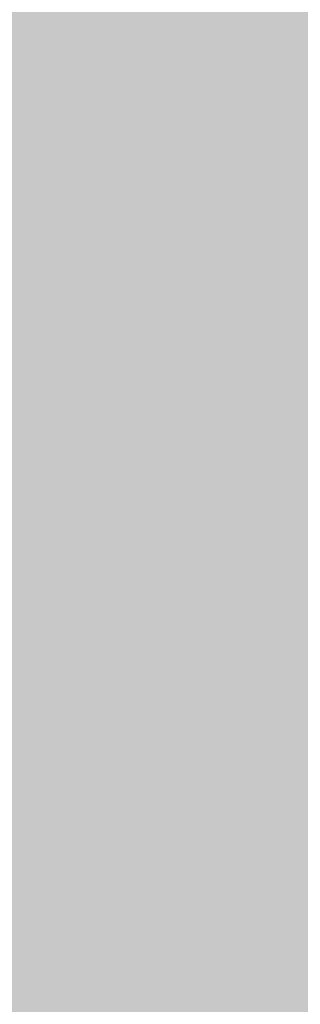
# Model space of a CAD drawing. Units: inches. Extents: x 2083 to 3317, y 1141 to 2115.
# Tile 178 of 256: x 3126.92826 to 3126.94671, y 1263.29018 to 1263.35483. Entities that reach past the tile are written whole.
import ezdxf

# ---------------------------------------------------------------- set-up
doc = ezdxf.new("R2010")
doc.units = ezdxf.units.IN
doc.layers.add('A-ANNO-DIMS', color=2, linetype='Continuous', lineweight=18)
doc.layers.add('A-WALL-PATT', color=251, linetype='Continuous', lineweight=13, true_color=0x636466)
doc.styles.get("Standard").update_dxf_attribs({"font": 'arial.ttf'})
doc.dimstyles.new('ISO-25', dxfattribs={"dimtxt": 12, "dimasz": 12, "dimexe": 1.25, "dimexo": 0.625, "dimtad": 1, "dimlunit": 3, "dimtxsty": 'Standard', "dimcen": 2.5, "dimadec": 0, "dimazin": 0, "dimtfac": 1, "dimtmove": 0, "dimatfit": 3, "dimfxl": 1, "dimarcsym": 0})

# ---------------------------------------------------------------- blocks, each defined once
blk = doc.blocks.new('*D26')
at = {"layer": 'A-ANNO-DIMS', "color": 0, "lineweight": -2, "transparency": 16777216}
for p, q in [((3088.985844, 1274.915092), (3088.985844, 1270.951963)), ((3111.240037, 1274.915092), (3111.240037, 1270.951963)), ((3076.985844, 1272.201963), (2840.262447, 1272.201963)), ((3111.240037, 1272.201963), (3088.985844, 1272.201963)), ((3123.240037, 1272.201963), (3135.240037, 1272.201963))]:
    blk.add_line(p, q, dxfattribs=at)
at = {"layer": 'A-ANNO-DIMS', "color": 0, "transparency": 16777216}
for points in [[(3076.985844, 1274.201963), (3076.985844, 1270.201963), (3088.985844, 1272.201963)], [(3123.240037, 1274.201963), (3123.240037, 1270.201963), (3111.240037, 1272.201963)]]:
    blk.add_solid(points, dxfattribs=at)
at = {"layer": 'Defpoints', "color": 0, "transparency": 16777216}
for p in [(3088.985844, 1275.540092), (3111.240037, 1275.540092), (3088.985844, 1272.201963)]:
    blk.add_point(p, dxfattribs=at)
at = {"layer": 'A-ANNO-DIMS', "color": 0, "transparency": 16777216, "insert": (2952.624146, 1279.031602), "char_height": 12, "attachment_point": 5}
blk.add_mtext('NIGHTSTAND 1\'-10 1/2" TYP.', dxfattribs=at)
blk = doc.blocks.new('*D27')
at = {"layer": 'A-ANNO-DIMS', "color": 0, "lineweight": -2, "transparency": 16777216}
for p, q in [((3114.578165, 1309.794285), (3114.578165, 1321.794285)), ((3111.865037, 1297.794285), (3115.828165, 1297.794285)), ((3114.578165, 1297.794285), (3114.578165, 1275.540092)), ((3111.865037, 1275.540092), (3115.828165, 1275.540092)), ((3114.578165, 1263.540092), (3114.578165, 1140.988591))]:
    blk.add_line(p, q, dxfattribs=at)
at = {"layer": 'A-ANNO-DIMS', "color": 0, "transparency": 16777216}
for points in [[(3112.578165, 1309.794285), (3116.578165, 1309.794285), (3114.578165, 1297.794285)], [(3112.578165, 1263.540092), (3116.578165, 1263.540092), (3114.578165, 1275.540092)]]:
    blk.add_solid(points, dxfattribs=at)
at = {"layer": 'Defpoints', "color": 0, "transparency": 16777216}
for p in [(3111.240037, 1297.794285), (3111.240037, 1275.540092), (3114.578165, 1275.540092)]:
    blk.add_point(p, dxfattribs=at)
at = {"layer": 'A-ANNO-DIMS', "color": 0, "transparency": 16777216, "insert": (3107.748527, 1196.264342), "char_height": 12, "attachment_point": 5, "rotation": 90}
blk.add_mtext('1\'-10 1/2" TYP.', dxfattribs=at)

msp = doc.modelspace()

# ---------------------------------------------------------------- hatches: boundary and pattern name
at = {"layer": 'A-WALL-PATT'}
h = msp.add_hatch(color=256, dxfattribs=at)
h.dxf.hatch_style = 1
h.paths.add_polyline_path([(3126.959783, 2020.76136), (2748.959783, 2020.76136), (2604.959783, 2020.76136), (2226.959783, 2020.76136), (2226.959783, 1702.76136), (2466.959783, 1702.76136), (2466.959783, 1582.76136), (2418.959783, 1582.76136), (2418.959783, 1477.76136), (2226.959783, 1477.76136), (2226.959783, 1263.26136), (2544.959783, 1263.26136), (2544.959783, 1411.76136), (2604.959783, 1411.76136), (2685.959783, 1411.76136), (2685.959783, 1420.76136), (2604.959783, 1420.76136), (2604.959783, 1573.76136), (2604.959783, 1702.76136), (2604.959783, 2011.76136), (2748.959783, 2011.76136), (2748.959783, 1702.76136), (2862.959783, 1702.76136), (2862.959783, 1621.76136), (2871.959783, 1621.76136), (2871.959783, 1702.76136), (2883.959783, 1702.76136), (2883.959783, 1706.939459, -0.026459), (2883.959783, 1711.76136), (2757.959783, 1711.76136), (2757.959783, 1807.76136), (2787.959783, 1807.76136), (2787.959783, 1812.26136), (2757.959783, 1812.26136), (2757.959783, 2011.76136), (2877.959783, 2011.76136), (2877.959783, 1812.26136), (2847.959783, 1812.26136), (2847.959783, 1807.76136), (2889.835742, 1807.76136), (2889.835742, 1812.26136), (2882.459783, 1812.26136), (2882.459783, 2011.76136), (3117.959783, 2011.76136), (3117.959783, 1812.26136), (2937.835742, 1812.26136), (2937.835742, 1807.76136), (2995.709783, 1807.76136), (2995.709783, 1796.117666), (3000.209783, 1796.117666), (3000.209783, 1807.76136), (3117.959783, 1807.76136), (3117.959783, 1711.76136), (3000.209783, 1711.76136), (3000.209783, 1760.117666), (2998.572705, 1760.117666, -0.020711), (2995.709783, 1760.117666), (2995.709783, 1711.76136), (2931.959783, 1711.76136), (2931.959783, 1702.76136), (3126.959783, 1702.76136)])
h.paths.add_polyline_path([(2471.459783, 2011.76136), (2471.459783, 1810.01136), (2462.716936, 1810.01136), (2462.716936, 1805.51136), (2505.959783, 1805.51136), (2505.959783, 1810.01136), (2475.959783, 1810.01136), (2475.959783, 2011.76136), (2595.959783, 2011.76136), (2595.959783, 1810.01136), (2565.959783, 1810.01136), (2565.959783, 1805.51136), (2595.959783, 1805.51136), (2595.959783, 1711.76136), (2235.959783, 1711.76136), (2235.959783, 1805.51136), (2353.709783, 1805.51136), (2353.709783, 1796.054162), (2358.209783, 1796.054162), (2358.209783, 1805.51136), (2414.716936, 1805.51136), (2414.716936, 1810.01136), (2235.959783, 1810.01136), (2235.959783, 2011.76136)], flags=16)
h.paths.add_polyline_path([(2270.204734, 1994.610008), (2270.204734, 1970.610008), (2246.204734, 1970.610008), (2246.204734, 1994.610008)], flags=0)
edge = h.paths.add_edge_path(flags=0)
edge.add_ellipse((2332.027391, 1899.798176), major_axis=(-3.042994, 3.042994), ratio=0.16825245, start_angle=-161.332166, end_angle=-156.307114, ccw=False)
edge.add_ellipse((2333.082037, 1898.74353), major_axis=(-1.054646, 1.054646), ratio=0.4535321, start_angle=-123.371019, end_angle=-94.159107)
edge = h.paths.add_edge_path(flags=0)
edge.add_ellipse((2332.027391, 1968.87629), major_axis=(3.042994, 3.042994), ratio=0.16825245, start_angle=18.667834, end_angle=23.692886)
edge.add_spline(control_points=[(2332.925596, 1970.691105), (2332.226768, 1970.3361), (2330.893709, 1969.658905), (2328.41308, 1970.932138), (2327.203934, 1967.748712), (2324.709596, 1969.955589), (2322.532822, 1967.012354), (2320.012846, 1971.295812), (2317.680308, 1968.157845), (2316.040526, 1967.102047), (2315.426904, 1966.809602)], knot_values=[0, 0, 0, 0, 2.267059, 4.324559, 6.685584, 8.878641, 11.121502, 14.300359, 17.755284, 19.732645, 19.732645, 19.732645, 19.732645], degree=3, periodic=0)
edge.add_ellipse((2332.027391, 1968.87629), major_axis=(3.042994, 3.042994), ratio=0.16825245, start_angle=18.667834, end_angle=23.692886, ccw=False)
edge.add_ellipse((2333.082037, 1969.930936), major_axis=(1.054646, 1.054646), ratio=0.4535321, start_angle=56.628981, end_angle=85.840893, ccw=False)
edge = h.paths.add_edge_path(flags=0)
edge.add_spline(control_points=[(2296.428287, 1967.987908), (2293.627804, 1965.336314), (2287.703624, 1959.727094), (2299.74386, 1949.995699), (2294.532591, 1935.668528), (2290.573228, 1920.603512), (2293.394124, 1909.973691), (2296.185407, 1904.966543)], knot_values=[0.099185, 0.099185, 0.099185, 0.099185, 0.345301, 0.619822, 0.982653, 1.386093, 1.810555, 1.810555, 1.810555, 1.810555], degree=3, periodic=0)
edge.add_spline(control_points=[(2296.185407, 1904.966543), (2297.383582, 1902.6193), (2298.000969, 1901.949312), (2298.55297, 1901.468155)], knot_values=[0.006246, 0.006246, 0.006246, 0.006246, 0.055476, 0.055476, 0.055476, 0.055476], degree=3, periodic=0)
edge.add_spline(control_points=[(2298.55297, 1901.468155), (2297.258612, 1900.923224), (2295.225294, 1900.232126), (2293.060229, 1900.614205), (2292.101423, 1900.788415), (2292.089578, 1900.790568)], knot_values=[0.312835, 0.312835, 0.312835, 0.312835, 0.40178, 0.474987, 0.475903, 0.475903, 0.475903, 0.475903], degree=3, periodic=0)
edge.add_arc((2292.793646, 1904.664109), 3.937008, 215.420897, 259.698179, ccw=False)
edge.add_spline(control_points=[(2289.585314, 1902.382304), (2289.476652, 1902.535087), (2289.36848, 1902.688035), (2289.260865, 1902.84117)], knot_values=[0.102872, 0.102872, 0.102872, 0.102872, 0.116896, 0.116896, 0.116896, 0.116896], degree=3, periodic=0)
edge.add_spline(control_points=[(2289.260865, 1902.84117), (2288.686604, 1902.550192), (2287.640048, 1902.019902), (2285.881337, 1901.873954), (2283.852972, 1901.504352), (2281.719987, 1899.710538), (2278.466991, 1899.492942), (2276.157136, 1901.883202), (2272.258953, 1899.804071), (2267.777605, 1901.843183), (2262.243882, 1900.184033), (2257.414927, 1901.782061), (2254.318374, 1900.72612), (2253.178285, 1900.337343)], knot_values=[0, 0, 0, 0, 1.907977, 3.477176, 5.261074, 7.972851, 11.680248, 13.717921, 16.939592, 22.789562, 27.502503, 33.595215, 37.145618, 37.145618, 37.145618, 37.145618], degree=3, periodic=0)
edge.add_line((2253.178285, 1900.337343), (2250.24424, 1902.84117))
edge.add_line((2250.24424, 1902.84117), (2250.24424, 1965.833296))
edge.add_line((2250.24424, 1965.833296), (2253.178285, 1968.337123))
edge.add_spline(control_points=[(2253.178285, 1968.337123), (2254.318374, 1967.948346), (2257.414927, 1966.892405), (2262.243882, 1968.490433), (2267.777605, 1966.831283), (2271.52673, 1968.537217), (2273.875914, 1967.828289), (2274.206701, 1967.727642)], knot_values=[0, 0, 0, 0, 0.09018, 0.244935, 0.364644, 0.513233, 0.537855, 0.537855, 0.537855, 0.537855], degree=3, periodic=0)
edge.add_arc((2274.352887, 1963.793349), 3.937008, 72.051134, 92.127949, ccw=False)
edge.add_arc((2281.296933, 1985.230003), 18.596298, 252.0511336, 288.5657217)
edge.add_arc((2292.316717, 1956.02888), 12.646081, 71.0267879, 113.7782184, ccw=False)
edge = h.paths.add_edge_path(flags=0)
edge.add_spline(control_points=[(2274.899415, 1951.856195), (2275.066156, 1951.616592), (2275.232687, 1951.376588), (2275.397987, 1951.135855)], knot_values=[1.409916, 1.409916, 1.409916, 1.409916, 1.43159, 1.43159, 1.43159, 1.43159], degree=3, periodic=0)
edge.add_spline(control_points=[(2275.397987, 1951.135855), (2275.792106, 1950.561885), (2276.179231, 1949.983774), (2276.545546, 1949.397103)], knot_values=[1.358238, 1.358238, 1.358238, 1.358238, 1.409916, 1.409916, 1.409916, 1.409916], degree=3, periodic=0)
edge.add_line((2276.545546, 1949.397103), (2277.437289, 1947.862185))
edge.add_spline(control_points=[(2277.437289, 1947.862185), (2276.303834, 1945.673115), (2274.639698, 1942.426882), (2274.631615, 1938.0939), (2272.799124, 1930.85155), (2274.356426, 1943.897046), (2275.947681, 1947.923356), (2276.545546, 1949.397103)], knot_values=[0.005632, 0.005632, 0.005632, 0.005632, 0.186014, 0.266002, 0.357087, 0.59639, 0.739732, 0.739732, 0.739732, 0.739732], degree=3, periodic=0)
edge.add_spline(control_points=[(2276.545546, 1949.397103), (2276.179231, 1949.983774), (2275.792106, 1950.561885), (2275.397987, 1951.135855)], knot_values=[1.358238, 1.358238, 1.358238, 1.358238, 1.409916, 1.409916, 1.409916, 1.409916], degree=3, periodic=0)
edge.add_spline(control_points=[(2275.397987, 1951.135855), (2274.9425, 1950.080452), (2274.20776, 1948.025272), (2273.934602, 1944.851477), (2272.468534, 1937.627489), (2273.466216, 1945.696466), (2274.700615, 1951.059472), (2274.899415, 1951.856195)], knot_values=[0.104364, 0.104364, 0.104364, 0.104364, 0.189636, 0.269624, 0.36071, 0.600013, 0.644622, 0.644622, 0.644622, 0.644622], degree=3, periodic=0)
h.paths.add_polyline_path([(2269.167514, 1963.127573, -0.357527), (2268.170633, 1960.97637, -0.092561), (2268.170633, 1939.436325, -0.357527), (2269.167514, 1937.285122, -0.357527), (2267.01631, 1938.282002, -0.164785), (2254.685581, 1938.282002, -0.357527), (2252.534378, 1937.285122, -0.357527), (2253.531259, 1939.436325, -0.092561), (2253.531259, 1960.97637, -0.357527), (2252.534378, 1963.127573, -0.357527), (2254.685581, 1962.130692, -0.164785), (2267.01631, 1962.130692, -0.357527)], flags=0)
h.paths.add_polyline_path([(2248.874068, 1967.8018), (2248.874068, 1957.02771), (2249.457783, 1957.02771), (2249.457783, 1911.646756), (2248.874068, 1911.646756), (2248.874068, 1900.872666), (2246.511863, 1900.872666, 0.197327), (2244.149658, 1902.456873), (2244.149658, 1966.217592, 0.197327), (2246.511863, 1967.8018)], flags=0)
h.paths.add_polyline_path([(2269.167514, 1931.389344, -0.357527), (2268.170633, 1929.238141, -0.092561), (2268.170633, 1907.698096, -0.357527), (2269.167514, 1905.546893, -0.357527), (2267.01631, 1906.543774, -0.164785), (2254.685581, 1906.543774, -0.357527), (2252.534378, 1905.546893, -0.357527), (2253.531259, 1907.698096, -0.092561), (2253.531259, 1929.238141, -0.357527), (2252.534378, 1931.389344, -0.357527), (2254.685581, 1930.392463, -0.164785), (2267.01631, 1930.392463, -0.357527)], flags=0)
edge = h.paths.add_edge_path(flags=0)
edge.add_spline(control_points=[(2276.196858, 1906.723702), (2276.168144, 1909.028928), (2276.114049, 1913.371852), (2270.598417, 1924.924978), (2273.905175, 1919.012779), (2275.921711, 1916.262063), (2275.47457, 1912.402149), (2277.257874, 1910.380621), (2276.696044, 1908.225036), (2276.646218, 1906.813023), (2276.617825, 1906.008407)], knot_values=[0, 0, 0, 0, 8.61026, 16.221274, 18.843057, 23.804898, 27.440828, 29.356102, 31.203478, 33.650687, 33.650687, 33.650687, 33.650687], degree=3, periodic=0)
edge.add_spline(control_points=[(2276.617825, 1906.008407), (2276.623313, 1905.624144), (2276.497738, 1904.628661), (2275.441779, 1903.854725), (2274.937314, 1903.08045), (2274.85908, 1902.84117)], knot_values=[0.156488, 0.156488, 0.156488, 0.156488, 0.184398, 0.231376, 0.250598, 0.250598, 0.250598, 0.250598], degree=3, periodic=0)
edge.add_line((2274.85908, 1902.84117), (2276.50598, 1902.84117))
edge.add_spline(control_points=[(2276.50598, 1902.84117), (2276.788308, 1903.08494), (2277.665071, 1904.125196), (2278.249538, 1904.340738), (2277.653872, 1908.527387), (2278.15567, 1906.227808), (2278.100464, 1905.285948), (2278.846675, 1904.069005), (2277.856785, 1903.414948), (2277.874191, 1902.99105), (2277.903562, 1902.84117)], knot_values=[0.059574, 0.059574, 0.059574, 0.059574, 0.080753, 0.103741, 0.16972, 0.176036, 0.207137, 0.240474, 0.262341, 0.27366, 0.27366, 0.27366, 0.27366], degree=3, periodic=0)
edge.add_line((2277.903562, 1902.84117), (2280.029825, 1902.84117))
edge.add_spline(control_points=[(2280.029825, 1902.84117), (2279.888221, 1903.088398), (2279.499257, 1903.981551), (2280.152284, 1905.939349), (2278.103615, 1909.657757), (2279.762395, 1907.185285), (2280.3279, 1904.874861), (2280.485109, 1903.48959), (2281.463269, 1903.249432), (2281.758343, 1902.936497), (2281.834036, 1902.84117)], knot_values=[0.013856, 0.013856, 0.013856, 0.013856, 0.034874, 0.088867, 0.107879, 0.126738, 0.158714, 0.193757, 0.217487, 0.226722, 0.226722, 0.226722, 0.226722], degree=3, periodic=0)
edge.add_spline(control_points=[(2281.834036, 1902.84117), (2281.787535, 1902.826703), (2281.647022, 1902.782988), (2281.395527, 1902.85949), (2281.088077, 1902.985242), (2280.720683, 1903.060902), (2280.333451, 1903.025726), (2280.124767, 1902.898879), (2280.029825, 1902.84117)], knot_values=[0, 0, 0, 0, 0.14413, 0.435517, 0.749276, 1.153046, 1.548371, 1.878348, 1.878348, 1.878348, 1.878348], degree=3, periodic=0)
edge.add_line((2280.029825, 1902.84117), (2277.903562, 1902.84117))
edge.add_spline(control_points=[(2277.903562, 1902.84117), (2277.892855, 1902.795855), (2277.865396, 1902.679637), (2277.607479, 1902.687483), (2277.27405, 1902.8007), (2276.837921, 1902.619775), (2276.583807, 1902.789261), (2276.50598, 1902.84117)], knot_values=[0, 0, 0, 0, 0.127189, 0.326199, 0.628009, 1.24357, 1.515331, 1.515331, 1.515331, 1.515331], degree=3, periodic=0)
edge.add_line((2276.50598, 1902.84117), (2274.85908, 1902.84117))
edge.add_spline(control_points=[(2274.85908, 1902.84117), (2274.814437, 1902.898587), (2274.72513, 1903.013446), (2274.493477, 1903.118968), (2274.244285, 1902.960539), (2273.937121, 1903.184942), (2273.614039, 1902.983143), (2273.408316, 1902.883045), (2273.322254, 1902.84117)], knot_values=[0, 0, 0, 0, 0.21843, 0.436957, 0.687977, 0.990379, 1.398396, 1.69185, 1.69185, 1.69185, 1.69185], degree=3, periodic=0)
edge.add_spline(control_points=[(2273.322254, 1902.84117), (2273.61674, 1903.445692), (2274.273998, 1904.538253), (2276.027239, 1904.573702), (2276.206963, 1906.583637), (2276.196858, 1906.723702)], knot_values=[0.012227, 0.012227, 0.012227, 0.012227, 0.059472, 0.106218, 0.134458, 0.134458, 0.134458, 0.134458], degree=3, periodic=0)
h.paths.add_polyline_path([(2270.776054, 1897.789828), (2270.776054, 1873.789828), (2246.776054, 1873.789828), (2246.776054, 1897.789828)], flags=0)
h.paths.add_polyline_path([(2353.709783, 1760.005059), (2353.709783, 1760.054162), (2358.209783, 1760.054162, -0.033729)], flags=0)
h.paths.add_polyline_path([(2321.819119, 1737.529186), (2341.995327, 1737.529186, -0.414214), (2343.203273, 1736.321241), (2343.203273, 1721.020596, -0.414214), (2341.995327, 1719.812651), (2321.819119, 1719.812651, -0.414214), (2320.611173, 1721.020596), (2320.611173, 1736.321241, -0.414214)], flags=0)
h.paths.add_polyline_path([(2324.23501, 1736.321241), (2339.579436, 1736.321241, -0.414214), (2341.995327, 1733.905349), (2341.995327, 1725.44973, -0.414214), (2339.579436, 1723.033839), (2333.680588, 1723.033839), (2333.845317, 1722.045467, -0.870646), (2335.425399, 1721.825893, -0.767327), (2333.922694, 1721.423245), (2331.291024, 1721.423245, -0.767327), (2329.788319, 1721.825893, -0.870646), (2331.368401, 1722.045467), (2331.53313, 1723.033839), (2324.23501, 1723.033839, -0.414214), (2321.819119, 1725.44973), (2321.819119, 1733.905349, -0.414214)], flags=0)
h.paths.add_polyline_path([(2570.483789, 1928.615444), (2589.683789, 1928.615444), (2590.168829, 1928.615444), (2590.168829, 1904.993397), (2570.483789, 1904.993397)], flags=0)
h.paths.add_polyline_path([(2574.447324, 1927.263822, -1), (2572.828836, 1927.263822, -1)], flags=0)
h.paths.add_polyline_path([(2573.089867, 1926.940877), (2573.925032, 1927.776042), (2574.147743, 1927.553332), (2573.312577, 1926.718166)], flags=0)
h.paths.add_polyline_path([(2578.779065, 1919.729618, -1), (2571.591663, 1919.729618, -1)], flags=0)
h.paths.add_polyline_path([(2578.385364, 1919.729618, -1), (2571.985364, 1919.729618, -1)], flags=0)
h.paths.add_polyline_path([(2331.595764, 1729.476216, -1), (2333.617954, 1729.476216, -1)], flags=0)
h.paths.add_polyline_path([(2578.034228, 1927.263822, -1), (2576.41574, 1927.263822, -1)], flags=0)
h.paths.add_polyline_path([(2576.688851, 1927.531089), (2576.911562, 1927.753799), (2577.746728, 1926.918634), (2577.524017, 1926.695923)], flags=0)
h.paths.add_polyline_path([(2578.139065, 1909.859539, -1), (2572.231663, 1909.859539, -1)], flags=0)
h.paths.add_polyline_path([(2577.745364, 1909.859539, -1), (2572.625364, 1909.859539, -1)], flags=0)
h.paths.add_polyline_path([(2583.797718, 1927.263822, -1), (2582.179229, 1927.263822, -1)], flags=0)
h.paths.add_polyline_path([(2582.718649, 1927.753799), (2583.553814, 1926.918634), (2583.331103, 1926.695923), (2582.495938, 1927.531089)], flags=0)
h.paths.add_polyline_path([(2582.495938, 1927.531089), (2582.718649, 1927.753799), (2583.553814, 1926.918634), (2583.331103, 1926.695923)], flags=0)
h.paths.add_polyline_path([(2587.739065, 1920.529618, -1), (2581.831663, 1920.529618, -1)], flags=0)
h.paths.add_polyline_path([(2587.345364, 1920.529618, -1), (2582.225364, 1920.529618, -1)], flags=0)
h.paths.add_polyline_path([(2587.384622, 1927.263822, -1), (2585.766133, 1927.263822, -1)], flags=0)
h.paths.add_polyline_path([(2586.081993, 1926.980247), (2586.917158, 1927.815412), (2587.139869, 1927.592702), (2586.304703, 1926.757536)], flags=0)
h.paths.add_polyline_path([(2588.379065, 1910.659539, -1), (2581.191663, 1910.659539, -1)], flags=0)
h.paths.add_polyline_path([(2587.985364, 1910.659539, -1), (2581.585364, 1910.659539, -1)], flags=0)
h.paths.add_polyline_path([(2417.167729, 1729.477895), (2437.343937, 1729.477895, -0.414214), (2438.551883, 1728.26995), (2438.551883, 1712.969306, -0.414214), (2437.343937, 1711.76136), (2417.167729, 1711.76136, -0.414214), (2415.959783, 1712.969306), (2415.959783, 1728.26995, -0.414214)], flags=0)
h.paths.add_polyline_path([(2419.58362, 1728.26995), (2434.928046, 1728.26995, -0.414214), (2437.343937, 1725.854059), (2437.343937, 1717.39844, -0.414214), (2434.928046, 1714.982548), (2429.029199, 1714.982548), (2429.193927, 1713.994176, -0.870646), (2430.774009, 1713.774603, -0.767327), (2429.271304, 1713.371954), (2426.639634, 1713.371954, -0.767327), (2425.136929, 1713.774603, -0.870646), (2426.717011, 1713.994176), (2426.88174, 1714.982548), (2419.58362, 1714.982548, -0.414214), (2417.167729, 1717.39844), (2417.167729, 1725.854059, -0.414214)], flags=0)
h.paths.add_polyline_path([(2419.58362, 1728.26995), (2434.928046, 1728.26995, -0.414214), (2437.343937, 1725.854059), (2437.343937, 1717.39844, -0.414214), (2434.928046, 1714.982548), (2429.029199, 1714.982548), (2428.358118, 1719.009034), (2427.552821, 1719.009034), (2426.88174, 1714.982548), (2419.58362, 1714.982548, -0.414214), (2417.167729, 1717.39844), (2417.167729, 1725.854059, -0.414214)], flags=0)
h.paths.add_polyline_path([(2426.944374, 1721.424925, -1), (2428.966564, 1721.424925, -1)], flags=0)
h.paths.add_polyline_path([(2475.959783, 1702.76136), (2595.959783, 1702.76136), (2595.959783, 1582.76136), (2475.959783, 1582.76136)], flags=16)
h.paths.add_polyline_path([(2427.959783, 1573.76136), (2595.959783, 1573.76136), (2595.959783, 1468.76136), (2595.959783, 1420.76136), (2384.459783, 1420.76136), (2384.459783, 1468.76136), (2427.959783, 1468.76136)], flags=16)
h.paths.add_polyline_path([(2379.959783, 1468.76136), (2379.959783, 1420.76136), (2235.959783, 1420.76136), (2235.959783, 1468.76136)], flags=16)
h.paths.add_polyline_path([(2317.815996, 1466.695767), (2337.992205, 1466.695767, -0.414214), (2339.20015, 1465.487821), (2339.20015, 1450.187177, -0.414214), (2337.992205, 1448.979232), (2317.815996, 1448.979232, -0.414214), (2316.608051, 1450.187177), (2316.608051, 1465.487821, -0.414214)], flags=0)
h.paths.add_polyline_path([(2320.231887, 1465.487821), (2335.576313, 1465.487821, -0.414214), (2337.992205, 1463.07193), (2337.992205, 1454.616311, -0.414214), (2335.576313, 1452.20042), (2329.677466, 1452.20042), (2329.842195, 1451.212047, -0.870646), (2331.422276, 1450.992474, -0.767327), (2329.919571, 1450.589826), (2327.287902, 1450.589826, -0.767327), (2325.785197, 1450.992474, -0.870646), (2327.365278, 1451.212047), (2327.530007, 1452.20042), (2320.231887, 1452.20042, -0.414214), (2317.815996, 1454.616311), (2317.815996, 1463.07193, -0.414214)], flags=0)
h.paths.add_polyline_path([(2320.231887, 1465.487821), (2335.576313, 1465.487821, -0.414214), (2337.992205, 1463.07193), (2337.992205, 1454.616311, -0.414214), (2335.576313, 1452.20042), (2329.677466, 1452.20042), (2329.006385, 1456.226905), (2328.201088, 1456.226905), (2327.530007, 1452.20042), (2320.231887, 1452.20042, -0.414214), (2317.815996, 1454.616311), (2317.815996, 1463.07193, -0.414214)], flags=0)
h.paths.add_polyline_path([(2327.592641, 1458.642796, -1), (2329.614832, 1458.642796, -1)], flags=0)
h.paths.add_polyline_path([(2244.411744, 1433.340453), (2241.920945, 1433.340453, -0.414214), (2240.017856, 1435.243542), (2240.017856, 1440.952808, -0.414211), (2241.920925, 1442.855897), (2244.411744, 1442.855897, -1.976472)], flags=0)
h.paths.add_polyline_path([(2245.356888, 1434.397536, -0.414214), (2245.356888, 1441.798814, -2.144098)], flags=0)
h.paths.add_polyline_path([(2535.959783, 1416.26136), (2535.959783, 1272.26136), (2235.959783, 1272.26136), (2235.959783, 1416.26136)], flags=16)
h.paths.add_polyline_path([(2260.119561, 1384.292841), (2260.119561, 1362.038649), (2237.865369, 1362.038649), (2237.865369, 1384.292841)], flags=0)
edge = h.paths.add_edge_path(flags=0)
edge.add_line((2318.251847, 1362.093298), (2318.145797, 1362.000973))
edge.add_ellipse((2317.445116, 1360.431044), major_axis=(2.82164, 2.82164), ratio=0.16825245, start_angle=18.667834, end_angle=20.948127, ccw=False)
edge.add_ellipse((2318.423045, 1361.408974), major_axis=(0.977929, 0.977929), ratio=0.4535321, start_angle=56.628981, end_angle=70.226201, ccw=False)
edge = h.paths.add_edge_path(flags=0)
edge.add_line((2319.10737, 1295.571078), (2319.015044, 1295.677128))
edge.add_ellipse((2317.445116, 1296.377809), major_axis=(-2.82164, 2.82164), ratio=0.16825245, start_angle=-161.332166, end_angle=-159.051873, ccw=False)
edge.add_ellipse((2318.423045, 1295.39988), major_axis=(-0.977929, 0.977929), ratio=0.4535321, start_angle=-123.371019, end_angle=-109.773799)
edge = h.paths.add_edge_path(flags=0)
edge.add_spline(control_points=[(2284.210349, 1301.170219), (2284.580688, 1300.444719), (2284.891189, 1299.892024), (2285.159553, 1299.461018)], knot_values=[0.039066, 0.039066, 0.039066, 0.039066, 0.055476, 0.055476, 0.055476, 0.055476], degree=3, periodic=0)
edge.add_line((2285.159553, 1299.461018), (2284.210349, 1301.170219))
edge = h.paths.add_edge_path(flags=0)
edge.add_line((2280.412458, 1297.298013), (2283.369991, 1297.036122))
edge.add_line((2283.369991, 1297.036122), (2286.40569, 1297.92631))
edge.add_spline(control_points=[(2286.40569, 1297.92631), (2285.305487, 1297.463119), (2284.344777, 1297.129151), (2283.369991, 1297.036122)], knot_values=[0.394369, 0.394369, 0.394369, 0.394369, 0.475903, 0.475903, 0.475903, 0.475903], degree=3, periodic=0)
edge.add_spline(control_points=[(2283.369991, 1297.036122), (2283.28139, 1297.027666), (2282.316289, 1296.957336), (2281.312502, 1297.134479), (2280.423441, 1297.296016), (2280.412458, 1297.298013)], knot_values=[0.312835, 0.312835, 0.312835, 0.312835, 0.320246, 0.393453, 0.394369, 0.394369, 0.394369, 0.394369], degree=3, periodic=0)
edge = h.paths.add_edge_path(flags=0)
edge.add_line((2284.435561, 1359.607285), (2280.446291, 1355.328047))
edge.add_line((2280.446291, 1355.328047), (2279.579987, 1351.017754))
edge.add_line((2279.579987, 1351.017754), (2282.412974, 1346.580433))
edge.add_spline(control_points=[(2282.412974, 1346.580433), (2283.153331, 1345.589236), (2284.252896, 1344.028897), (2284.801037, 1342.387167), (2284.935162, 1341.805544)], knot_values=[1.240098, 1.240098, 1.240098, 1.240098, 1.332892, 1.382712, 1.382712, 1.382712, 1.382712], degree=3, periodic=0)
edge.add_spline(control_points=[(2284.935162, 1341.805544), (2285.319108, 1340.1406), (2285.233029, 1338.409204), (2284.909938, 1336.654122)], knot_values=[1.097484, 1.097484, 1.097484, 1.097484, 1.240098, 1.240098, 1.240098, 1.240098], degree=3, periodic=0)
edge.add_spline(control_points=[(2284.909938, 1336.654122), (2284.586848, 1334.89904), (2284.026745, 1333.120272), (2283.462644, 1331.360585)], knot_values=[0.95487, 0.95487, 0.95487, 0.95487, 1.097484, 1.097484, 1.097484, 1.097484], degree=3, periodic=0)
edge.add_line((2283.462644, 1331.360585), (2281.890376, 1326.153357))
edge.add_line((2281.890376, 1326.153357), (2280.756259, 1321.056089))
edge.add_line((2280.756259, 1321.056089), (2280.299205, 1316.001977))
edge.add_line((2280.299205, 1316.001977), (2280.715933, 1310.950068))
edge.add_line((2280.715933, 1310.950068), (2282.028094, 1305.972137))
edge.add_line((2282.028094, 1305.972137), (2284.210349, 1301.170219))
edge.add_spline(control_points=[(2284.210349, 1301.170219), (2283.340731, 1302.730185), (2282.611904, 1304.336493), (2282.028094, 1305.972137)], knot_values=[0.099185, 0.099185, 0.099185, 0.099185, 0.241799, 0.241799, 0.241799, 0.241799], degree=3, periodic=0)
edge.add_spline(control_points=[(2282.028094, 1305.972137), (2281.444283, 1307.60778), (2281.005489, 1309.272759), (2280.715933, 1310.950068)], knot_values=[0.241799, 0.241799, 0.241799, 0.241799, 0.384413, 0.384413, 0.384413, 0.384413], degree=3, periodic=0)
edge.add_spline(control_points=[(2280.715933, 1310.950068), (2280.433241, 1312.587613), (2280.289386, 1314.276959), (2280.298894, 1315.962032), (2280.299205, 1316.001977)], knot_values=[0.384413, 0.384413, 0.384413, 0.384413, 0.523647, 0.527028, 0.527028, 0.527028, 0.527028], degree=3, periodic=0)
edge.add_spline(control_points=[(2280.299205, 1316.001977), (2280.312326, 1317.686955), (2280.477871, 1319.367926), (2280.756259, 1321.056089)], knot_values=[0.527028, 0.527028, 0.527028, 0.527028, 0.669642, 0.669642, 0.669642, 0.669642], degree=3, periodic=0)
edge.add_spline(control_points=[(2280.756259, 1321.056089), (2281.034648, 1322.744252), (2281.42588, 1324.439608), (2281.890376, 1326.153357)], knot_values=[0.669642, 0.669642, 0.669642, 0.669642, 0.812256, 0.812256, 0.812256, 0.812256], degree=3, periodic=0)
edge.add_spline(control_points=[(2281.890376, 1326.153357), (2282.264383, 1327.533251), (2282.78787, 1329.26181), (2283.352751, 1331.01778), (2283.462644, 1331.360585)], knot_values=[0.812256, 0.812256, 0.812256, 0.812256, 0.927087, 0.95487, 0.95487, 0.95487, 0.95487], degree=3, periodic=0)
edge.add_line((2283.462644, 1331.360585), (2284.909938, 1336.654122))
edge.add_line((2284.909938, 1336.654122), (2284.935162, 1341.805544))
edge.add_line((2284.935162, 1341.805544), (2282.412974, 1346.580433))
edge.add_spline(control_points=[(2282.412974, 1346.580433), (2281.275127, 1348.103792), (2280.078447, 1349.570318), (2279.579987, 1351.017754)], knot_values=[1.382712, 1.382712, 1.382712, 1.382712, 1.525326, 1.525326, 1.525326, 1.525326], degree=3, periodic=0)
edge.add_spline(control_points=[(2279.579987, 1351.017754), (2279.443282, 1351.414721), (2279.136312, 1352.856922), (2279.73519, 1354.290385), (2280.446291, 1355.328047)], knot_values=[1.525326, 1.525326, 1.525326, 1.525326, 1.564439, 1.667941, 1.667941, 1.667941, 1.667941], degree=3, periodic=0)
edge.add_spline(control_points=[(2280.446291, 1355.328047), (2281.426113, 1356.757835), (2282.930837, 1358.18256), (2284.435561, 1359.607285)], knot_values=[1.667941, 1.667941, 1.667941, 1.667941, 1.810555, 1.810555, 1.810555, 1.810555], degree=3, periodic=0)
edge.add_arc((2280.623075, 1348.518181), 11.72618, 71.0267879, 113.7782184)
edge.add_arc((2270.404892, 1375.595156), 17.243567, 252.0511336, 288.5657217, ccw=False)
edge.add_arc((2263.965969, 1355.717847), 3.650622, 72.051134, 92.127949)
edge.add_arc((2263.965969, 1355.717847), 3.650622, 92.127949, 177.98513)
edge.add_spline(control_points=[(2260.317604, 1355.846199), (2260.260417, 1354.220668), (2260.551278, 1350.186547), (2262.999344, 1346.766251), (2264.472741, 1344.649024)], knot_values=[1.43159, 1.43159, 1.43159, 1.43159, 1.564144, 1.770695, 1.770695, 1.770695, 1.770695], degree=3, periodic=0)
edge.add_line((2264.472741, 1344.649024), (2264.93559, 1343.98253))
edge.add_spline(control_points=[(2263.801044, 1340.248105), (2263.843238, 1340.514088), (2264.067244, 1341.756465), (2264.512693, 1343.002453), (2264.935047, 1343.981083)], knot_values=[0.53657, 0.53657, 0.53657, 0.53657, 0.559349, 0.644622, 0.644622, 0.644622, 0.644622], degree=3, periodic=0)
edge.add_spline(control_points=[(2264.935047, 1343.981083), (2265.117771, 1343.714975), (2265.298875, 1343.447906), (2265.476756, 1343.179365)], knot_values=[1.384077, 1.384077, 1.384077, 1.384077, 1.409916, 1.409916, 1.409916, 1.409916], degree=3, periodic=0)
edge.add_spline(control_points=[(2265.476756, 1343.179365), (2265.654637, 1342.910823), (2265.829296, 1342.64081), (2265.99913, 1342.368812)], knot_values=[1.358238, 1.358238, 1.358238, 1.358238, 1.384077, 1.384077, 1.384077, 1.384077], degree=3, periodic=0)
edge.add_line((2265.99913, 1342.368812), (2266.826006, 1340.945547))
edge.add_spline(control_points=[(2266.826006, 1340.945547), (2268.894401, 1337.089691), (2271.398173, 1325.843001), (2270.516164, 1310.568557), (2275.919376, 1301.860609), (2277.789511, 1299.19945)], knot_values=[0.116896, 0.116896, 0.116896, 0.116896, 0.472987, 1.050969, 1.313793, 1.313793, 1.313793, 1.313793], degree=3, periodic=0)
edge.add_spline(control_points=[(2277.789511, 1299.19945), (2277.839405, 1299.128452), (2277.889428, 1299.057498), (2277.939572, 1298.986584)], knot_values=[0.109884, 0.109884, 0.109884, 0.109884, 0.116896, 0.116896, 0.116896, 0.116896], degree=3, periodic=0)
edge.add_line((2277.939572, 1298.986584), (2277.788849, 1299.199114))
edge.add_spline(control_points=[(2277.788849, 1299.199114), (2277.256582, 1298.929414), (2276.28635, 1298.437902), (2275.039352, 1298.334419), (2274.38333, 1298.238895), (2274.215254, 1298.209338)], knot_values=[33.12187, 33.12187, 33.12187, 33.12187, 35.029056, 36.598255, 37.144827, 37.144827, 37.144827, 37.144827], degree=3, periodic=0)
edge.add_line((2274.215254, 1298.209338), (2273.073147, 1297.892961))
edge.add_spline(control_points=[(2273.073147, 1297.892961), (2272.322936, 1297.579784), (2271.039151, 1296.510508), (2269.248395, 1296.226062), (2268.4231, 1296.374654)], knot_values=[26.532584, 26.532584, 26.532584, 26.532584, 29.198919, 31.839101, 31.839101, 31.839101, 31.839101], degree=3, periodic=0)
edge.add_line((2268.4231, 1296.374654), (2263.878501, 1297.457534))
edge.add_spline(control_points=[(2263.878501, 1297.457534), (2263.556077, 1297.359435), (2261.860306, 1296.838694), (2260.23878, 1297.282407), (2258.933454, 1297.516461)], knot_values=[15.919551, 15.919551, 15.919551, 15.919551, 16.939592, 21.226067, 21.226067, 21.226067, 21.226067], degree=3, periodic=0)
edge.add_line((2258.933454, 1297.516461), (2254.055233, 1297.32901))
edge.add_spline(control_points=[(2254.055233, 1297.32901), (2253.755525, 1297.295815), (2252.113683, 1297.165174), (2250.461869, 1297.544221), (2249.129686, 1297.667882)], knot_values=[5.306517, 5.306517, 5.306517, 5.306517, 6.276435, 10.613034, 10.613034, 10.613034, 10.613034], degree=3, periodic=0)
edge.add_line((2249.129686, 1297.667882), (2244.33165, 1296.877756))
edge.add_line((2244.33165, 1296.877756), (2241.611033, 1299.19945))
edge.add_line((2241.611033, 1299.19945), (2241.611033, 1357.609404))
edge.add_line((2241.611033, 1357.609404), (2244.33165, 1359.931097))
edge.add_line((2244.33165, 1359.931097), (2252.728823, 1359.542692))
edge.add_spline(control_points=[(2252.728823, 1359.542692), (2252.870939, 1359.54644), (2253.30574, 1359.548172), (2253.739845, 1359.514274), (2254.031742, 1359.482426)], knot_values=[0.233291, 0.233291, 0.233291, 0.233291, 0.244935, 0.268927, 0.268927, 0.268927, 0.268927], degree=3, periodic=0)
edge.add_line((2254.031742, 1359.482426), (2259.58719, 1359.41639))
edge.add_spline(control_points=[(2259.58719, 1359.41639), (2260.677068, 1359.628503), (2262.073197, 1359.897003), (2263.523692, 1359.459278), (2263.830417, 1359.365952)], knot_values=[0.422516, 0.422516, 0.422516, 0.422516, 0.513233, 0.537855, 0.537855, 0.537855, 0.537855], degree=3, periodic=0)
edge.add_arc((2263.965969, 1355.717847), 3.650622, 72.051134, 92.127949, ccw=False)
edge.add_arc((2270.404892, 1375.595156), 17.243567, 252.0511336, 288.5657217)
edge.add_arc((2280.623075, 1348.518181), 11.72618, 71.0267879, 113.7782184, ccw=False)
h.paths.add_polyline_path([(2240.34053, 1359.434715), (2240.34053, 1349.444353), (2240.881785, 1349.444353), (2240.881785, 1307.3645), (2240.34053, 1307.3645), (2240.34053, 1297.374138), (2238.150157, 1297.374138, 0.197327), (2235.959783, 1298.843108), (2235.959783, 1357.965746, 0.197327), (2238.150157, 1359.434715)], flags=0)
h.paths.add_polyline_path([(2259.15779, 1355.1005, -0.357527), (2258.233425, 1353.10578, -0.092561), (2258.233425, 1333.132601, -0.357527), (2259.15779, 1331.13788, -0.357527), (2257.16307, 1332.062246, -0.164785), (2245.729302, 1332.062246, -0.357527), (2243.734582, 1331.13788, -0.357527), (2244.658947, 1333.132601, -0.092561), (2244.658947, 1353.10578, -0.357527), (2243.734582, 1355.1005, -0.357527), (2245.729302, 1354.176135, -0.164785), (2257.16307, 1354.176135, -0.357527)], flags=0)
edge = h.paths.add_edge_path(flags=0)
edge.add_line((2265.99913, 1342.368812), (2266.826006, 1340.945547))
edge.add_line((2266.826006, 1340.945547), (2265.307557, 1337.814066))
edge.add_line((2265.307557, 1337.814066), (2264.358232, 1334.652939))
edge.add_line((2264.358232, 1334.652939), (2264.262012, 1333.799705))
edge.add_spline(control_points=[(2264.262012, 1333.799705), (2264.208357, 1333.187055), (2264.16206, 1332.365525), (2264.007144, 1331.413933), (2263.969049, 1331.201834)], knot_values=[0.464444, 0.464444, 0.464444, 0.464444, 0.516691, 0.531608, 0.531608, 0.531608, 0.531608], degree=3, periodic=0)
edge.add_spline(control_points=[(2263.969049, 1331.201834), (2263.774535, 1330.118873), (2263.42437, 1328.790839), (2263.25742, 1328.530652), (2263.234028, 1328.514612)], knot_values=[0.372682, 0.372682, 0.372682, 0.372682, 0.44885, 0.464444, 0.464444, 0.464444, 0.464444], degree=3, periodic=0)
edge.add_spline(control_points=[(2263.234028, 1328.514612), (2263.096382, 1328.420227), (2263.13117, 1329.301477), (2263.274953, 1330.615749)], knot_values=[0.280919, 0.280919, 0.280919, 0.280919, 0.372682, 0.372682, 0.372682, 0.372682], degree=3, periodic=0)
edge.add_spline(control_points=[(2263.274953, 1330.615749), (2263.418736, 1331.930022), (2263.671515, 1333.677318), (2263.969852, 1335.315027)], knot_values=[0.189157, 0.189157, 0.189157, 0.189157, 0.280919, 0.280919, 0.280919, 0.280919], degree=3, periodic=0)
edge.add_spline(control_points=[(2263.969852, 1335.315027), (2264.100496, 1336.032192), (2264.418783, 1337.621911), (2264.754848, 1338.86443), (2264.947419, 1339.491124)], knot_values=[0.097394, 0.097394, 0.097394, 0.097394, 0.137578, 0.189157, 0.189157, 0.189157, 0.189157], degree=3, periodic=0)
edge.add_spline(control_points=[(2264.947419, 1339.491124), (2265.290017, 1340.606055), (2265.644238, 1341.493996), (2265.99913, 1342.368812)], knot_values=[0.005632, 0.005632, 0.005632, 0.005632, 0.097394, 0.097394, 0.097394, 0.097394], degree=3, periodic=0)
h.paths.add_polyline_path([(2259.15779, 1325.670973, -0.357527), (2258.233425, 1323.676253, -0.092561), (2258.233425, 1303.703073, -0.357527), (2259.15779, 1301.708353, -0.357527), (2257.16307, 1302.632719, -0.164785), (2245.729302, 1302.632719, -0.357527), (2243.734582, 1301.708353, -0.357527), (2244.658947, 1303.703073, -0.092561), (2244.658947, 1323.676253, -0.357527), (2243.734582, 1325.670973, -0.357527), (2245.729302, 1324.746608, -0.164785), (2257.16307, 1324.746608, -0.357527)], flags=0)
edge = h.paths.add_edge_path(flags=0)
edge.add_spline(control_points=[(2261.708938, 1317.311421), (2261.679482, 1317.41758), (2261.761858, 1317.388535), (2262.490736, 1316.089873), (2262.962185, 1315.300897)], knot_values=[14.955861, 14.955861, 14.955861, 14.955861, 16.221274, 18.694826, 18.694826, 18.694826, 18.694826], degree=3, periodic=0)
edge.add_spline(control_points=[(2262.962185, 1315.300897), (2262.990437, 1315.253617), (2263.702096, 1314.067376), (2264.348983, 1313.127153), (2264.730054, 1312.164154)], knot_values=[18.694826, 18.694826, 18.694826, 18.694826, 18.843057, 22.433791, 22.433791, 22.433791, 22.433791], degree=3, periodic=0)
edge.add_spline(control_points=[(2264.730054, 1312.164154), (2264.875565, 1311.796437), (2265.176873, 1310.769807), (2265.143069, 1309.559262), (2265.247736, 1308.824193)], knot_values=[22.433791, 22.433791, 22.433791, 22.433791, 23.804898, 26.172756, 26.172756, 26.172756, 26.172756], degree=3, periodic=0)
edge.add_line((2265.247736, 1308.824193), (2265.850774, 1307.171888))
edge.add_spline(control_points=[(2265.850774, 1307.171888), (2266.065025, 1306.821678), (2266.384387, 1306.332246), (2266.4244, 1305.780549), (2266.420369, 1305.611216)], knot_values=[28.062562, 28.062562, 28.062562, 28.062562, 29.356102, 29.911721, 29.911721, 29.911721, 29.911721], degree=3, periodic=0)
edge.add_spline(control_points=[(2266.420369, 1305.611216), (2266.416116, 1305.43259), (2266.393999, 1305.249998), (2266.364777, 1305.065857)], knot_values=[29.911721, 29.911721, 29.911721, 29.911721, 30.497837, 30.497837, 30.497837, 30.497837], degree=3, periodic=0)
edge.add_line((2266.364777, 1305.065857), (2266.066151, 1302.136295))
edge.add_spline(control_points=[(2266.066151, 1302.136295), (2266.07124, 1301.779984), (2265.998076, 1301.199985), (2265.663266, 1300.758961), (2265.508908, 1300.585882)], knot_values=[0.156488, 0.156488, 0.156488, 0.156488, 0.184398, 0.203543, 0.203543, 0.203543, 0.203543], degree=3, periodic=0)
edge.add_line((2265.508908, 1300.585882), (2264.435341, 1299.19945))
edge.add_line((2264.435341, 1299.19945), (2265.962442, 1299.19945))
edge.add_line((2265.962442, 1299.19945), (2267.33599, 1301.175276))
edge.add_line((2267.33599, 1301.175276), (2267.311667, 1301.986237))
edge.add_spline(control_points=[(2267.311667, 1301.986237), (2267.261111, 1302.862396), (2267.160212, 1303.737132), (2267.271486, 1303.325896)], knot_values=[0.126229, 0.126229, 0.126229, 0.126229, 0.166617, 0.166617, 0.166617, 0.166617], degree=3, periodic=0)
edge.add_spline(control_points=[(2267.271486, 1303.325896), (2267.280035, 1303.294305), (2267.309785, 1303.175366), (2267.37345, 1302.883608), (2267.406123, 1302.682829), (2267.417926, 1302.601025)], knot_values=[0.166617, 0.166617, 0.166617, 0.166617, 0.16972, 0.176036, 0.180765, 0.180765, 0.180765, 0.180765], degree=3, periodic=0)
edge.add_spline(control_points=[(2267.743891, 1300.987505), (2267.687583, 1301.150943), (2267.48052, 1301.656664), (2267.483751, 1302.144788), (2267.417926, 1302.601025)], knot_values=[0.180765, 0.180765, 0.180765, 0.180765, 0.193767, 0.220139, 0.220139, 0.220139, 0.220139], degree=3, periodic=0)
edge.add_line((2267.417926, 1302.601025), (2267.743891, 1300.987505))
edge.add_spline(control_points=[(2267.743891, 1300.987505), (2267.831961, 1300.731878), (2267.932021, 1300.309904), (2267.554841, 1299.974518), (2267.429366, 1299.829207)], knot_values=[0.220139, 0.220139, 0.220139, 0.220139, 0.240474, 0.25489, 0.25489, 0.25489, 0.25489], degree=3, periodic=0)
edge.add_line((2267.429366, 1299.829207), (2267.258361, 1299.19945))
edge.add_line((2267.258361, 1299.19945), (2269.229956, 1299.19945))
edge.add_spline(control_points=[(2269.229956, 1299.19945), (2269.098653, 1299.428694), (2268.842774, 1300.016251), (2269.011575, 1300.915923), (2268.946796, 1301.66074)], knot_values=[0.013856, 0.013856, 0.013856, 0.013856, 0.034874, 0.067073, 0.067073, 0.067073, 0.067073], degree=3, periodic=0)
edge.add_line((2268.946796, 1301.66074), (2268.431582, 1303.603109))
edge.add_spline(control_points=[(2268.431582, 1303.603109), (2268.175596, 1304.192375), (2267.596214, 1305.251298), (2268.040698, 1304.62321), (2268.251394, 1304.282421)], knot_values=[0.090155, 0.090155, 0.090155, 0.090155, 0.107879, 0.120289, 0.120289, 0.120289, 0.120289], degree=3, periodic=0)
edge.add_spline(control_points=[(2268.251394, 1304.282421), (2268.360882, 1304.105329), (2269.057753, 1302.917983), (2269.382691, 1301.590419), (2269.521405, 1300.775931), (2269.57522, 1300.555784)], knot_values=[0.120289, 0.120289, 0.120289, 0.120289, 0.126738, 0.158714, 0.173506, 0.173506, 0.173506, 0.173506], degree=3, periodic=0)
edge.add_line((2269.57522, 1300.555784), (2270.685798, 1299.421258))
edge.add_spline(control_points=[(2270.685798, 1299.421258), (2270.767221, 1299.357251), (2270.837852, 1299.281401), (2270.902925, 1299.19945)], knot_values=[0.21816, 0.21816, 0.21816, 0.21816, 0.226722, 0.226722, 0.226722, 0.226722], degree=3, periodic=0)
edge.add_line((2270.937201, 1299.192913), (2270.902925, 1299.19945))
edge.add_spline(control_points=[(2270.902925, 1299.19945), (2270.859806, 1299.186035), (2270.729515, 1299.1455), (2270.496314, 1299.216437), (2270.271661, 1299.308323), (2270.121017, 1299.347961), (2270.063339, 1299.359557)], knot_values=[0.939174, 0.939174, 0.939174, 0.939174, 1.083304, 1.374691, 1.68845, 1.878348, 1.878348, 1.878348, 1.878348], degree=3, periodic=0)
edge.add_line((2270.063339, 1299.359557), (2269.229956, 1299.19945))
edge.add_line((2269.229956, 1299.19945), (2267.258361, 1299.19945))
edge.add_spline(control_points=[(2267.258361, 1299.19945), (2267.248433, 1299.157431), (2267.222971, 1299.049667), (2266.983816, 1299.056942), (2266.80921, 1299.11623), (2266.676905, 1299.109091), (2266.636531, 1299.104815)], knot_values=[0.757665, 0.757665, 0.757665, 0.757665, 0.884854, 1.083864, 1.385675, 1.515331, 1.515331, 1.515331, 1.515331], degree=3, periodic=0)
edge.add_spline(control_points=[(2266.636531, 1299.104815), (2266.485225, 1299.088788), (2266.235807, 1299.017123), (2266.034608, 1299.151317), (2265.962442, 1299.19945)], knot_values=[0, 0, 0, 0, 0.485905, 0.757665, 0.757665, 0.757665, 0.757665], degree=3, periodic=0)
edge.add_line((2265.962442, 1299.19945), (2264.435341, 1299.19945))
edge.add_line((2264.435341, 1299.19945), (2263.858444, 1299.367118))
edge.add_spline(control_points=[(2263.858444, 1299.367118), (2263.818943, 1299.370905), (2263.779528, 1299.385721), (2263.740131, 1299.401504)], knot_values=[0.845925, 0.845925, 0.845925, 0.845925, 0.978627, 0.978627, 0.978627, 0.978627], degree=3, periodic=0)
edge.add_line((2263.721786, 1299.396425), (2263.010306, 1299.19945))
edge.add_spline(control_points=[(2263.010306, 1299.19945), (2263.245794, 1299.682859), (2263.506032, 1300.128107), (2263.873494, 1300.408028)], knot_values=[0.012227, 0.012227, 0.012227, 0.012227, 0.052971, 0.052971, 0.052971, 0.052971], degree=3, periodic=0)
edge.add_spline(control_points=[(2263.873494, 1300.408028), (2263.932131, 1300.452695), (2264.084243, 1300.552979), (2264.255189, 1300.624223), (2264.359686, 1300.664747)], knot_values=[0.052971, 0.052971, 0.052971, 0.052971, 0.059472, 0.069086, 0.069086, 0.069086, 0.069086], degree=3, periodic=0)
edge.add_line((2264.359686, 1300.664747), (2265.1419, 1301.077774))
edge.add_line((2265.1419, 1301.077774), (2265.675806, 1302.799558))
edge.add_line((2265.675806, 1302.799558), (2265.5407, 1305.704066))
edge.add_line((2265.5407, 1305.704066), (2264.803073, 1309.327724))
edge.add_line((2264.803073, 1309.327724), (2263.040535, 1314.091791))
edge.add_spline(control_points=[(2263.040535, 1314.091791), (2262.383572, 1315.671438), (2261.795972, 1316.997749), (2261.708938, 1317.311421)], knot_values=[11.216896, 11.216896, 11.216896, 11.216896, 14.955861, 14.955861, 14.955861, 14.955861], degree=3, periodic=0)
h.paths.add_polyline_path([(2871.959783, 1416.26136), (2895.910047, 1416.26136), (2895.910047, 1420.76136), (2871.959783, 1420.76136), (2871.959783, 1501.76136), (2862.959783, 1501.76136), (2862.959783, 1420.76136), (2805.959783, 1420.76136), (2805.959783, 1411.76136), (2862.959783, 1411.76136), (2862.959783, 1263.26136), (3126.959783, 1263.26136), (3126.959783, 1411.76136), (3126.959783, 1486.76136), (2943.959783, 1486.76136), (2943.959783, 1477.76136), (2967.860311, 1477.76136), (2967.860311, 1420.76136), (2943.910047, 1420.76136), (2943.910047, 1416.26136), (3117.959783, 1416.26136), (3117.959783, 1420.76136), (2972.360311, 1420.76136), (2972.360311, 1477.76136), (3117.959783, 1477.76136), (3117.959783, 1420.76136), (3117.959783, 1272.26136), (2871.959783, 1272.26136)], flags=0)
h.paths.add_polyline_path([(2457.125626, 1485.942505), (2527.602651, 1485.942505), (2527.602651, 1537.635702), (2457.125626, 1537.635702)], flags=8)
h.paths.add_polyline_path([(2481.005058, 1609.981804), (2590.765818, 1609.981804), (2590.765818, 1682.003362), (2481.005058, 1682.003362)], flags=8)
h.paths.add_polyline_path([(2483.085022, 1729.126784), (2553.562048, 1729.126784), (2553.562048, 1780.81998), (2483.085022, 1780.81998)], flags=8)
h = msp.add_hatch(color=256, dxfattribs=at)
h.dxf.hatch_style = 1
h.paths.add_polyline_path([(3126.959783, 1486.76136), (2943.959783, 1486.76136), (2943.959783, 1477.76136), (2967.860311, 1477.76136), (2967.860311, 1420.76136), (2943.910047, 1420.76136), (2943.910047, 1416.26136), (3117.959783, 1416.26136), (3117.959783, 1420.76136), (2972.360311, 1420.76136), (2972.360311, 1477.76136), (3117.959783, 1477.76136), (3117.959783, 1420.76136), (3117.959783, 1272.26136), (2871.959783, 1272.26136), (2871.959783, 1416.26136), (2895.910047, 1416.26136), (2895.910047, 1420.76136), (2871.959783, 1420.76136), (2871.959783, 1501.76136), (2862.959783, 1501.76136), (2862.959783, 1420.76136), (2805.959783, 1420.76136), (2805.959783, 1411.76136), (2862.959783, 1411.76136), (2862.959783, 1263.26136), (3126.959783, 1263.26136), (3126.959783, 1411.76136)])

# ---------------------------------------------------------------- dimensions: what is measured, and where the dimension line sits
at = {"layer": 'A-ANNO-DIMS'}
for base, p1, p2, angle, text, picture, middle in [((3114.578165, 1275.540092), (3111.240037, 1297.794285), (3111.240037, 1275.540092), 270, '<> TYP.', '*D27', (3107.748527, 1196.264342)), ((3088.985844, 1272.201963), (3111.240037, 1275.540092), (3088.985844, 1275.540092), 180, 'NIGHTSTAND <> TYP.', '*D26', (2952.624146, 1279.031602))]:
    dim = msp.add_linear_dim(base=base, p1=p1, p2=p2, angle=angle, text=text, dimstyle='ISO-25', override={"dimdec": 1, "dimlfac": 1, "dimrnd": 0, "dimzin": 1, "dimdsep": 46, "dimlunit": 4, "dimfrac": 2}, dxfattribs=at)
    dim.commit()
    dim.dimension.update_dxf_attribs({"geometry": picture, "text_midpoint": middle})

doc.saveas('drawing.dxf')
